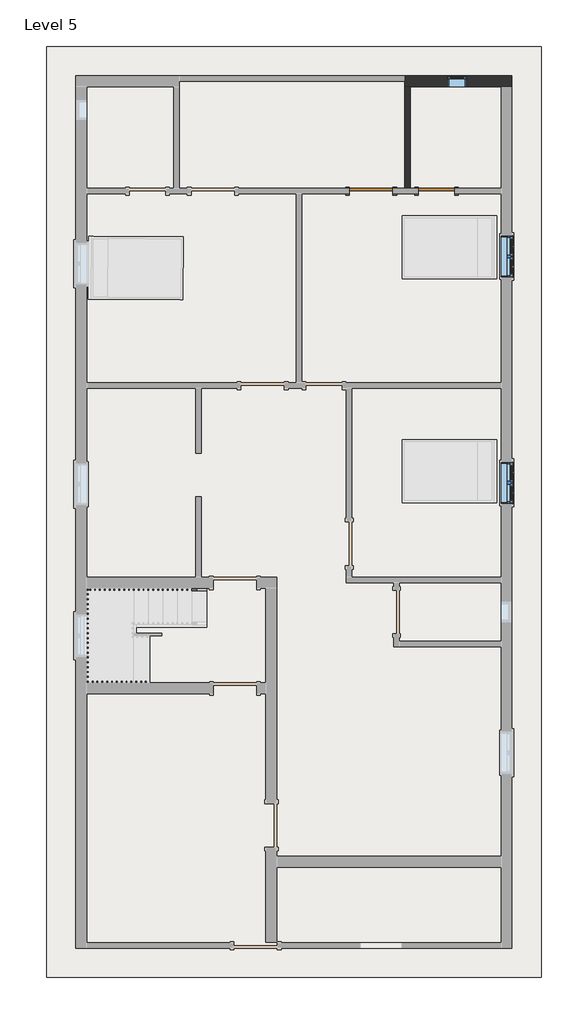
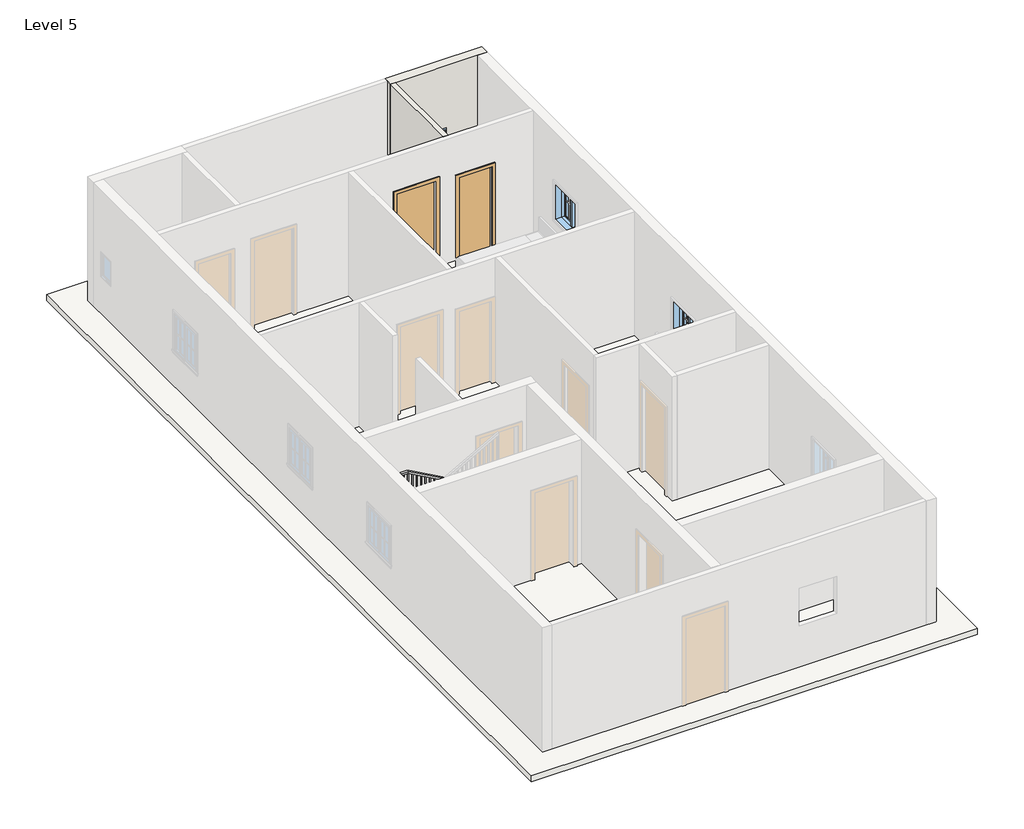
# One storey, part 2 of 3: 3 windows, 2 doors, 2 walls, 1 railing, 1 roof.
"""IFC4 building model written with IfcOpenShell, lengths in millimetres."""

from ifc_helpers import new_model, si_unit, frame, origin, place, context, project, spatial, polyline, outline, extrude, faceted_brep, transform, mapped, element, save
from components import door_f2b275c1, door_e5f9f3c4, window_aa618e30, window_339605e1

model = new_model("IFC4")

# Units and contexts
model_context = context("Model", 3, world=origin())
ifc_project = project(units=[si_unit("LENGTHUNIT", "METRE", prefix="MILLI")], contexts=[model_context])

# Site, building, storey
site = spatial("IfcSite", under=ifc_project)
building = spatial("IfcBuilding", under=site)
storey = spatial("IfcBuildingStorey", under=building, Name="Level 5", Elevation=9601.2)

# Doors
placement = place(None, origin())
door_shape = door_f2b275c1(model_context)
element("IfcDoor", 1, ObjectType="Single-Flush : 30\" x 80\"", at=placement, inside=storey, context=model_context, shape_type="MappedRepresentation", body=[
    mapped(door_shape, transform((1735.6084916, 8007.7072267, 9601.2), x_axis=(-1.0, 0.0, 0.0), y_axis=(0.0, -1.0, 0.0), z_axis=(0.0, 0.0, 1.0))),
])
door_2_shape = door_e5f9f3c4(model_context)
element("IfcDoor", 2, ObjectType="Single-Flush : 36\" x 84\"", at=placement, inside=storey, context=model_context, shape_type="MappedRepresentation", body=[
    mapped(door_2_shape, transform((364.0084916, 8007.7072267, 9601.2), x_axis=(1.0, 0.0, 0.0), y_axis=(0.0, 1.0, 0.0), z_axis=(0.0, 0.0, 1.0))),
])

# Railing
element("IfcRailing", 3, ObjectType="Handrail - Rectangular", at=placement, inside=storey, context=model_context, shape_type="SolidModel", body=[
    faceted_brep([(-3084.0415084, -367.9427733, 10684.9333333), (-3084.0415084, -367.9427733, 10626.820221), (-3084.0415084, -317.1427733, 10626.820221), (-3084.0415084, -317.1427733, 10684.9333333), (-4608.0415084, -367.9427733, 11531.6), (-4621.2051106, -367.9427733, 11480.8), (-4621.2051106, -317.1427733, 11480.8), (-4608.0415084, -317.1427733, 11531.6), (-5547.8415084, -367.9427733, 11531.6), (-5547.8415084, -367.9427733, 11480.8), (-5598.6415084, -317.1427733, 11480.8), (-5598.6415084, -317.1427733, 11531.6), (-5547.8415084, -2247.5427733, 11531.6), (-5547.8415084, -2247.5427733, 11480.8), (-5598.6415084, -2298.3427733, 11480.8), (-5598.6415084, -2298.3427733, 11531.6), (-4912.8415084, -2247.5427733, 11531.6), (-4899.6779062, -2247.5427733, 11480.8), (-4899.6779062, -2298.3427733, 11480.8), (-4912.8415084, -2298.3427733, 11531.6), (-3084.0415084, -2247.5427733, 12547.6), (-3084.0415084, -2298.3427733, 12547.6), (-3084.0415084, -2298.3427733, 12489.4868876), (-3084.0415084, -2247.5427733, 12489.4868876)], [[[0, 1, 2, 3]], [[1, 0, 4, 5]], [[2, 1, 5, 6]], [[3, 2, 6, 7]], [[0, 3, 7, 4]], [[5, 4, 8, 9]], [[6, 5, 9, 10]], [[7, 6, 10, 11]], [[4, 7, 11, 8]], [[9, 8, 12, 13]], [[10, 9, 13, 14]], [[11, 10, 14, 15]], [[8, 11, 15, 12]], [[13, 12, 16, 17]], [[14, 13, 17, 18]], [[15, 14, 18, 19]], [[12, 15, 19, 16]], [[20, 21, 22, 23]], [[17, 16, 20, 23]], [[18, 17, 23, 22]], [[19, 18, 22, 21]], [[16, 19, 21, 20]]]),
    extrude(outline(polyline([(12466.5563321, -3125.3165084), (12455.9729988, -3144.3665084), (11463.8666667, -3144.3665084), (11463.8666667, -3125.3165084), (12466.5563321, -3125.3165084)])), frame((0.0, -2282.4677733, 0.0), z_axis=(0.0, 1.0, 0.0), x_axis=(0.0, 0.0, 1.0)), (0.0, 0.0, 1.0), 19.05),
    extrude(outline(polyline([(12410.1118876, -3226.9165084), (12399.5285543, -3245.9665084), (11463.8666667, -3245.9665084), (11463.8666667, -3226.9165084), (12410.1118876, -3226.9165084)])), frame((0.0, -2282.4677733, 0.0), z_axis=(0.0, 1.0, 0.0), x_axis=(0.0, 0.0, 1.0)), (0.0, 0.0, 1.0), 19.05),
    extrude(outline(polyline([(12353.6674432, -3328.5165084), (12343.0841099, -3347.5665084), (11463.8666667, -3347.5665084), (11463.8666667, -3328.5165084), (12353.6674432, -3328.5165084)])), frame((0.0, -2282.4677733, 0.0), z_axis=(0.0, 1.0, 0.0), x_axis=(0.0, 0.0, 1.0)), (0.0, 0.0, 1.0), 19.05),
    extrude(outline(polyline([(12297.2229988, -3430.1165084), (12286.6396654, -3449.1665084), (11294.5333333, -3449.1665084), (11294.5333333, -3430.1165084), (12297.2229988, -3430.1165084)])), frame((0.0, -2282.4677733, 0.0), z_axis=(0.0, 1.0, 0.0), x_axis=(0.0, 0.0, 1.0)), (0.0, 0.0, 1.0), 19.05),
    extrude(outline(polyline([(12240.7785543, -3531.7165084), (12230.195221, -3550.7665084), (11294.5333333, -3550.7665084), (11294.5333333, -3531.7165084), (12240.7785543, -3531.7165084)])), frame((0.0, -2282.4677733, 0.0), z_axis=(0.0, 1.0, 0.0), x_axis=(0.0, 0.0, 1.0)), (0.0, 0.0, 1.0), 19.05),
    extrude(outline(polyline([(12184.3341099, -3633.3165084), (12173.7507765, -3652.3665084), (11294.5333333, -3652.3665084), (11294.5333333, -3633.3165084), (12184.3341099, -3633.3165084)])), frame((0.0, -2282.4677733, 0.0), z_axis=(0.0, 1.0, 0.0), x_axis=(0.0, 0.0, 1.0)), (0.0, 0.0, 1.0), 19.05),
    extrude(outline(polyline([(12127.8896654, -3734.9165084), (12117.3063321, -3753.9665084), (11125.2, -3753.9665084), (11125.2, -3734.9165084), (12127.8896654, -3734.9165084)])), frame((0.0, -2282.4677733, 0.0), z_axis=(0.0, 1.0, 0.0), x_axis=(0.0, 0.0, 1.0)), (0.0, 0.0, 1.0), 19.05),
    extrude(outline(polyline([(12071.445221, -3836.5165084), (12060.8618876, -3855.5665084), (11125.2, -3855.5665084), (11125.2, -3836.5165084), (12071.445221, -3836.5165084)])), frame((0.0, -2282.4677733, 0.0), z_axis=(0.0, 1.0, 0.0), x_axis=(0.0, 0.0, 1.0)), (0.0, 0.0, 1.0), 19.05),
    extrude(outline(polyline([(12015.0007765, -3938.1165084), (12004.4174432, -3957.1665084), (11125.2, -3957.1665084), (11125.2, -3938.1165084), (12015.0007765, -3938.1165084)])), frame((0.0, -2282.4677733, 0.0), z_axis=(0.0, 1.0, 0.0), x_axis=(0.0, 0.0, 1.0)), (0.0, 0.0, 1.0), 19.05),
    extrude(outline(polyline([(11958.5563321, -4039.7165084), (11947.9729988, -4058.7665084), (10955.8666667, -4058.7665084), (10955.8666667, -4039.7165084), (11958.5563321, -4039.7165084)])), frame((0.0, -2282.4677733, 0.0), z_axis=(0.0, 1.0, 0.0), x_axis=(0.0, 0.0, 1.0)), (0.0, 0.0, 1.0), 19.05),
    extrude(outline(polyline([(11902.1118876, -4141.3165084), (11891.5285543, -4160.3665084), (10955.8666667, -4160.3665084), (10955.8666667, -4141.3165084), (11902.1118876, -4141.3165084)])), frame((0.0, -2282.4677733, 0.0), z_axis=(0.0, 1.0, 0.0), x_axis=(0.0, 0.0, 1.0)), (0.0, 0.0, 1.0), 19.05),
    extrude(outline(polyline([(11845.6674432, -4242.9165084), (11835.0841099, -4261.9665084), (10955.8666667, -4261.9665084), (10955.8666667, -4242.9165084), (11845.6674432, -4242.9165084)])), frame((0.0, -2282.4677733, 0.0), z_axis=(0.0, 1.0, 0.0), x_axis=(0.0, 0.0, 1.0)), (0.0, 0.0, 1.0), 19.05),
    extrude(outline(polyline([(11789.2229988, -4344.5165084), (11778.6396654, -4363.5665084), (10786.5333333, -4363.5665084), (10786.5333333, -4344.5165084), (11789.2229988, -4344.5165084)])), frame((0.0, -2282.4677733, 0.0), z_axis=(0.0, 1.0, 0.0), x_axis=(0.0, 0.0, 1.0)), (0.0, 0.0, 1.0), 19.05),
    extrude(outline(polyline([(11732.7785543, -4446.1165084), (11722.195221, -4465.1665084), (10786.5333333, -4465.1665084), (10786.5333333, -4446.1165084), (11732.7785543, -4446.1165084)])), frame((0.0, -2282.4677733, 0.0), z_axis=(0.0, 1.0, 0.0), x_axis=(0.0, 0.0, 1.0)), (0.0, 0.0, 1.0), 19.05),
    extrude(outline(polyline([(11676.3341099, -4547.7165084), (11665.7507765, -4566.7665084), (10786.5333333, -4566.7665084), (10786.5333333, -4547.7165084), (11676.3341099, -4547.7165084)])), frame((0.0, -2282.4677733, 0.0), z_axis=(0.0, 1.0, 0.0), x_axis=(0.0, 0.0, 1.0)), (0.0, 0.0, 1.0), 19.05),
    extrude(outline(polyline([(11619.8896654, -4649.3165084), (11609.3063321, -4668.3665084), (10617.2, -4668.3665084), (10617.2, -4649.3165084), (11619.8896654, -4649.3165084)])), frame((0.0, -2282.4677733, 0.0), z_axis=(0.0, 1.0, 0.0), x_axis=(0.0, 0.0, 1.0)), (0.0, 0.0, 1.0), 19.05),
    extrude(outline(polyline([(11563.445221, -4750.9165084), (11552.8618876, -4769.9665084), (10617.2, -4769.9665084), (10617.2, -4750.9165084), (11563.445221, -4750.9165084)])), frame((0.0, -2282.4677733, 0.0), z_axis=(0.0, 1.0, 0.0), x_axis=(0.0, 0.0, 1.0)), (0.0, 0.0, 1.0), 19.05),
    extrude(outline(polyline([(11507.0007765, -4852.5165084), (11496.4174432, -4871.5665084), (10617.2, -4871.5665084), (10617.2, -4852.5165084), (11507.0007765, -4852.5165084)])), frame((0.0, -2282.4677733, 0.0), z_axis=(0.0, 1.0, 0.0), x_axis=(0.0, 0.0, 1.0)), (0.0, 0.0, 1.0), 19.05),
    extrude(outline(polyline([(-4973.1665084, -2282.4677733), (-4973.1665084, -2263.4177733), (-4954.1165084, -2263.4177733), (-4954.1165084, -2282.4677733), (-4973.1665084, -2282.4677733)])), frame((0.0, 0.0, 10617.2), z_axis=(0.0, 0.0, 1.0), x_axis=(1.0, 0.0, 0.0)), (0.0, 0.0, 1.0), 863.6),
    extrude(outline(polyline([(-5074.7665084, -2282.4677733), (-5074.7665084, -2263.4177733), (-5055.7165084, -2263.4177733), (-5055.7165084, -2282.4677733), (-5074.7665084, -2282.4677733)])), frame((0.0, 0.0, 10617.2), z_axis=(0.0, 0.0, 1.0), x_axis=(1.0, 0.0, 0.0)), (0.0, 0.0, 1.0), 863.6),
    extrude(outline(polyline([(-5176.3665084, -2282.4677733), (-5176.3665084, -2263.4177733), (-5157.3165084, -2263.4177733), (-5157.3165084, -2282.4677733), (-5176.3665084, -2282.4677733)])), frame((0.0, 0.0, 10617.2), z_axis=(0.0, 0.0, 1.0), x_axis=(1.0, 0.0, 0.0)), (0.0, 0.0, 1.0), 863.6),
    extrude(outline(polyline([(-5277.9665084, -2282.4677733), (-5277.9665084, -2263.4177733), (-5258.9165084, -2263.4177733), (-5258.9165084, -2282.4677733), (-5277.9665084, -2282.4677733)])), frame((0.0, 0.0, 10617.2), z_axis=(0.0, 0.0, 1.0), x_axis=(1.0, 0.0, 0.0)), (0.0, 0.0, 1.0), 863.6),
    extrude(outline(polyline([(-5379.5665084, -2282.4677733), (-5379.5665084, -2263.4177733), (-5360.5165084, -2263.4177733), (-5360.5165084, -2282.4677733), (-5379.5665084, -2282.4677733)])), frame((0.0, 0.0, 10617.2), z_axis=(0.0, 0.0, 1.0), x_axis=(1.0, 0.0, 0.0)), (0.0, 0.0, 1.0), 863.6),
    extrude(outline(polyline([(-5481.1665084, -2282.4677733), (-5481.1665084, -2263.4177733), (-5462.1165084, -2263.4177733), (-5462.1165084, -2282.4677733), (-5481.1665084, -2282.4677733)])), frame((0.0, 0.0, 10617.2), z_axis=(0.0, 0.0, 1.0), x_axis=(1.0, 0.0, 0.0)), (0.0, 0.0, 1.0), 863.6),
    extrude(outline(polyline([(-5582.7665084, -2161.8177733), (-5563.7165084, -2161.8177733), (-5563.7165084, -2180.8677733), (-5582.7665084, -2180.8677733), (-5582.7665084, -2161.8177733)])), frame((0.0, 0.0, 10617.2), z_axis=(0.0, 0.0, 1.0), x_axis=(1.0, 0.0, 0.0)), (0.0, 0.0, 1.0), 863.6),
    extrude(outline(polyline([(-5582.7665084, -2060.2177733), (-5563.7165084, -2060.2177733), (-5563.7165084, -2079.2677733), (-5582.7665084, -2079.2677733), (-5582.7665084, -2060.2177733)])), frame((0.0, 0.0, 10617.2), z_axis=(0.0, 0.0, 1.0), x_axis=(1.0, 0.0, 0.0)), (0.0, 0.0, 1.0), 863.6),
    extrude(outline(polyline([(-5582.7665084, -1958.6177733), (-5563.7165084, -1958.6177733), (-5563.7165084, -1977.6677733), (-5582.7665084, -1977.6677733), (-5582.7665084, -1958.6177733)])), frame((0.0, 0.0, 10617.2), z_axis=(0.0, 0.0, 1.0), x_axis=(1.0, 0.0, 0.0)), (0.0, 0.0, 1.0), 863.6),
    extrude(outline(polyline([(-5582.7665084, -1857.0177733), (-5563.7165084, -1857.0177733), (-5563.7165084, -1876.0677733), (-5582.7665084, -1876.0677733), (-5582.7665084, -1857.0177733)])), frame((0.0, 0.0, 10617.2), z_axis=(0.0, 0.0, 1.0), x_axis=(1.0, 0.0, 0.0)), (0.0, 0.0, 1.0), 863.6),
    extrude(outline(polyline([(-5582.7665084, -1755.4177733), (-5563.7165084, -1755.4177733), (-5563.7165084, -1774.4677733), (-5582.7665084, -1774.4677733), (-5582.7665084, -1755.4177733)])), frame((0.0, 0.0, 10617.2), z_axis=(0.0, 0.0, 1.0), x_axis=(1.0, 0.0, 0.0)), (0.0, 0.0, 1.0), 863.6),
    extrude(outline(polyline([(-5582.7665084, -1653.8177733), (-5563.7165084, -1653.8177733), (-5563.7165084, -1672.8677733), (-5582.7665084, -1672.8677733), (-5582.7665084, -1653.8177733)])), frame((0.0, 0.0, 10617.2), z_axis=(0.0, 0.0, 1.0), x_axis=(1.0, 0.0, 0.0)), (0.0, 0.0, 1.0), 863.6),
    extrude(outline(polyline([(-5582.7665084, -1552.2177733), (-5563.7165084, -1552.2177733), (-5563.7165084, -1571.2677733), (-5582.7665084, -1571.2677733), (-5582.7665084, -1552.2177733)])), frame((0.0, 0.0, 10617.2), z_axis=(0.0, 0.0, 1.0), x_axis=(1.0, 0.0, 0.0)), (0.0, 0.0, 1.0), 863.6),
    extrude(outline(polyline([(-5582.7665084, -1450.6177733), (-5563.7165084, -1450.6177733), (-5563.7165084, -1469.6677733), (-5582.7665084, -1469.6677733), (-5582.7665084, -1450.6177733)])), frame((0.0, 0.0, 10617.2), z_axis=(0.0, 0.0, 1.0), x_axis=(1.0, 0.0, 0.0)), (0.0, 0.0, 1.0), 863.6),
    extrude(outline(polyline([(-5582.7665084, -1349.0177733), (-5563.7165084, -1349.0177733), (-5563.7165084, -1368.0677733), (-5582.7665084, -1368.0677733), (-5582.7665084, -1349.0177733)])), frame((0.0, 0.0, 10617.2), z_axis=(0.0, 0.0, 1.0), x_axis=(1.0, 0.0, 0.0)), (0.0, 0.0, 1.0), 863.6),
    extrude(outline(polyline([(-5582.7665084, -1247.4177733), (-5563.7165084, -1247.4177733), (-5563.7165084, -1266.4677733), (-5582.7665084, -1266.4677733), (-5582.7665084, -1247.4177733)])), frame((0.0, 0.0, 10617.2), z_axis=(0.0, 0.0, 1.0), x_axis=(1.0, 0.0, 0.0)), (0.0, 0.0, 1.0), 863.6),
    extrude(outline(polyline([(-5582.7665084, -1145.8177733), (-5563.7165084, -1145.8177733), (-5563.7165084, -1164.8677733), (-5582.7665084, -1164.8677733), (-5582.7665084, -1145.8177733)])), frame((0.0, 0.0, 10617.2), z_axis=(0.0, 0.0, 1.0), x_axis=(1.0, 0.0, 0.0)), (0.0, 0.0, 1.0), 863.6),
    extrude(outline(polyline([(-5582.7665084, -1044.2177733), (-5563.7165084, -1044.2177733), (-5563.7165084, -1063.2677733), (-5582.7665084, -1063.2677733), (-5582.7665084, -1044.2177733)])), frame((0.0, 0.0, 10617.2), z_axis=(0.0, 0.0, 1.0), x_axis=(1.0, 0.0, 0.0)), (0.0, 0.0, 1.0), 863.6),
    extrude(outline(polyline([(-5582.7665084, -942.6177733), (-5563.7165084, -942.6177733), (-5563.7165084, -961.6677733), (-5582.7665084, -961.6677733), (-5582.7665084, -942.6177733)])), frame((0.0, 0.0, 10617.2), z_axis=(0.0, 0.0, 1.0), x_axis=(1.0, 0.0, 0.0)), (0.0, 0.0, 1.0), 863.6),
    extrude(outline(polyline([(-5582.7665084, -841.0177733), (-5563.7165084, -841.0177733), (-5563.7165084, -860.0677733), (-5582.7665084, -860.0677733), (-5582.7665084, -841.0177733)])), frame((0.0, 0.0, 10617.2), z_axis=(0.0, 0.0, 1.0), x_axis=(1.0, 0.0, 0.0)), (0.0, 0.0, 1.0), 863.6),
    extrude(outline(polyline([(-5582.7665084, -739.4177733), (-5563.7165084, -739.4177733), (-5563.7165084, -758.4677733), (-5582.7665084, -758.4677733), (-5582.7665084, -739.4177733)])), frame((0.0, 0.0, 10617.2), z_axis=(0.0, 0.0, 1.0), x_axis=(1.0, 0.0, 0.0)), (0.0, 0.0, 1.0), 863.6),
    extrude(outline(polyline([(-5582.7665084, -637.8177733), (-5563.7165084, -637.8177733), (-5563.7165084, -656.8677733), (-5582.7665084, -656.8677733), (-5582.7665084, -637.8177733)])), frame((0.0, 0.0, 10617.2), z_axis=(0.0, 0.0, 1.0), x_axis=(1.0, 0.0, 0.0)), (0.0, 0.0, 1.0), 863.6),
    extrude(outline(polyline([(-5582.7665084, -536.2177733), (-5563.7165084, -536.2177733), (-5563.7165084, -555.2677733), (-5582.7665084, -555.2677733), (-5582.7665084, -536.2177733)])), frame((0.0, 0.0, 10617.2), z_axis=(0.0, 0.0, 1.0), x_axis=(1.0, 0.0, 0.0)), (0.0, 0.0, 1.0), 863.6),
    extrude(outline(polyline([(-5582.7665084, -434.6177733), (-5563.7165084, -434.6177733), (-5563.7165084, -453.6677733), (-5582.7665084, -453.6677733), (-5582.7665084, -434.6177733)])), frame((0.0, 0.0, 10617.2), z_axis=(0.0, 0.0, 1.0), x_axis=(1.0, 0.0, 0.0)), (0.0, 0.0, 1.0), 863.6),
    extrude(outline(polyline([(-5512.9165084, -333.0177733), (-5512.9165084, -352.0677733), (-5531.9665084, -352.0677733), (-5531.9665084, -333.0177733), (-5512.9165084, -333.0177733)])), frame((0.0, 0.0, 10617.2), z_axis=(0.0, 0.0, 1.0), x_axis=(1.0, 0.0, 0.0)), (0.0, 0.0, 1.0), 863.6),
    extrude(outline(polyline([(-5411.3165084, -333.0177733), (-5411.3165084, -352.0677733), (-5430.3665084, -352.0677733), (-5430.3665084, -333.0177733), (-5411.3165084, -333.0177733)])), frame((0.0, 0.0, 10617.2), z_axis=(0.0, 0.0, 1.0), x_axis=(1.0, 0.0, 0.0)), (0.0, 0.0, 1.0), 863.6),
    extrude(outline(polyline([(-5309.7165084, -333.0177733), (-5309.7165084, -352.0677733), (-5328.7665084, -352.0677733), (-5328.7665084, -333.0177733), (-5309.7165084, -333.0177733)])), frame((0.0, 0.0, 10617.2), z_axis=(0.0, 0.0, 1.0), x_axis=(1.0, 0.0, 0.0)), (0.0, 0.0, 1.0), 863.6),
    extrude(outline(polyline([(-5208.1165084, -333.0177733), (-5208.1165084, -352.0677733), (-5227.1665084, -352.0677733), (-5227.1665084, -333.0177733), (-5208.1165084, -333.0177733)])), frame((0.0, 0.0, 10617.2), z_axis=(0.0, 0.0, 1.0), x_axis=(1.0, 0.0, 0.0)), (0.0, 0.0, 1.0), 863.6),
    extrude(outline(polyline([(-5106.5165084, -333.0177733), (-5106.5165084, -352.0677733), (-5125.5665084, -352.0677733), (-5125.5665084, -333.0177733), (-5106.5165084, -333.0177733)])), frame((0.0, 0.0, 10617.2), z_axis=(0.0, 0.0, 1.0), x_axis=(1.0, 0.0, 0.0)), (0.0, 0.0, 1.0), 863.6),
    extrude(outline(polyline([(-5004.9165084, -333.0177733), (-5004.9165084, -352.0677733), (-5023.9665084, -352.0677733), (-5023.9665084, -333.0177733), (-5004.9165084, -333.0177733)])), frame((0.0, 0.0, 10617.2), z_axis=(0.0, 0.0, 1.0), x_axis=(1.0, 0.0, 0.0)), (0.0, 0.0, 1.0), 863.6),
    extrude(outline(polyline([(-4903.3165084, -333.0177733), (-4903.3165084, -352.0677733), (-4922.3665084, -352.0677733), (-4922.3665084, -333.0177733), (-4903.3165084, -333.0177733)])), frame((0.0, 0.0, 10617.2), z_axis=(0.0, 0.0, 1.0), x_axis=(1.0, 0.0, 0.0)), (0.0, 0.0, 1.0), 863.6),
    extrude(outline(polyline([(-4801.7165084, -333.0177733), (-4801.7165084, -352.0677733), (-4820.7665084, -352.0677733), (-4820.7665084, -333.0177733), (-4801.7165084, -333.0177733)])), frame((0.0, 0.0, 10617.2), z_axis=(0.0, 0.0, 1.0), x_axis=(1.0, 0.0, 0.0)), (0.0, 0.0, 1.0), 863.6),
    extrude(outline(polyline([(-4700.1165084, -333.0177733), (-4700.1165084, -352.0677733), (-4719.1665084, -352.0677733), (-4719.1665084, -333.0177733), (-4700.1165084, -333.0177733)])), frame((0.0, 0.0, 10617.2), z_axis=(0.0, 0.0, 1.0), x_axis=(1.0, 0.0, 0.0)), (0.0, 0.0, 1.0), 863.6),
    extrude(outline(polyline([(11468.195221, -4598.5165084), (11478.7785543, -4617.5665084), (10617.2, -4617.5665084), (10617.2, -4598.5165084), (11468.195221, -4598.5165084)])), frame((0.0, -352.0677733, 0.0), z_axis=(0.0, 1.0, 0.0), x_axis=(0.0, 0.0, 1.0)), (0.0, 0.0, 1.0), 19.05),
    extrude(outline(polyline([(11411.7507765, -4496.9165084), (11422.3341099, -4515.9665084), (10447.8666667, -4515.9665084), (10447.8666667, -4496.9165084), (11411.7507765, -4496.9165084)])), frame((0.0, -352.0677733, 0.0), z_axis=(0.0, 1.0, 0.0), x_axis=(0.0, 0.0, 1.0)), (0.0, 0.0, 1.0), 19.05),
    extrude(outline(polyline([(11355.3063321, -4395.3165084), (11365.8896654, -4414.3665084), (10447.8666667, -4414.3665084), (10447.8666667, -4395.3165084), (11355.3063321, -4395.3165084)])), frame((0.0, -352.0677733, 0.0), z_axis=(0.0, 1.0, 0.0), x_axis=(0.0, 0.0, 1.0)), (0.0, 0.0, 1.0), 19.05),
    extrude(outline(polyline([(11298.8618876, -4293.7165084), (11309.445221, -4312.7665084), (10447.8666667, -4312.7665084), (10447.8666667, -4293.7165084), (11298.8618876, -4293.7165084)])), frame((0.0, -352.0677733, 0.0), z_axis=(0.0, 1.0, 0.0), x_axis=(0.0, 0.0, 1.0)), (0.0, 0.0, 1.0), 19.05),
    extrude(outline(polyline([(11242.4174432, -4192.1165084), (11253.0007765, -4211.1665084), (10278.5333333, -4211.1665084), (10278.5333333, -4192.1165084), (11242.4174432, -4192.1165084)])), frame((0.0, -352.0677733, 0.0), z_axis=(0.0, 1.0, 0.0), x_axis=(0.0, 0.0, 1.0)), (0.0, 0.0, 1.0), 19.05),
    extrude(outline(polyline([(11185.9729988, -4090.5165084), (11196.5563321, -4109.5665084), (10278.5333333, -4109.5665084), (10278.5333333, -4090.5165084), (11185.9729988, -4090.5165084)])), frame((0.0, -352.0677733, 0.0), z_axis=(0.0, 1.0, 0.0), x_axis=(0.0, 0.0, 1.0)), (0.0, 0.0, 1.0), 19.05),
    extrude(outline(polyline([(11129.5285543, -3988.9165084), (11140.1118876, -4007.9665084), (10278.5333333, -4007.9665084), (10278.5333333, -3988.9165084), (11129.5285543, -3988.9165084)])), frame((0.0, -352.0677733, 0.0), z_axis=(0.0, 1.0, 0.0), x_axis=(0.0, 0.0, 1.0)), (0.0, 0.0, 1.0), 19.05),
    extrude(outline(polyline([(11073.0841099, -3887.3165084), (11083.6674432, -3906.3665084), (10109.2, -3906.3665084), (10109.2, -3887.3165084), (11073.0841099, -3887.3165084)])), frame((0.0, -352.0677733, 0.0), z_axis=(0.0, 1.0, 0.0), x_axis=(0.0, 0.0, 1.0)), (0.0, 0.0, 1.0), 19.05),
    extrude(outline(polyline([(11016.6396654, -3785.7165084), (11027.2229988, -3804.7665084), (10109.2, -3804.7665084), (10109.2, -3785.7165084), (11016.6396654, -3785.7165084)])), frame((0.0, -352.0677733, 0.0), z_axis=(0.0, 1.0, 0.0), x_axis=(0.0, 0.0, 1.0)), (0.0, 0.0, 1.0), 19.05),
    extrude(outline(polyline([(10960.195221, -3684.1165084), (10970.7785543, -3703.1665084), (10109.2, -3703.1665084), (10109.2, -3684.1165084), (10960.195221, -3684.1165084)])), frame((0.0, -352.0677733, 0.0), z_axis=(0.0, 1.0, 0.0), x_axis=(0.0, 0.0, 1.0)), (0.0, 0.0, 1.0), 19.05),
    extrude(outline(polyline([(10903.7507765, -3582.5165084), (10914.3341099, -3601.5665084), (9939.8666667, -3601.5665084), (9939.8666667, -3582.5165084), (10903.7507765, -3582.5165084)])), frame((0.0, -352.0677733, 0.0), z_axis=(0.0, 1.0, 0.0), x_axis=(0.0, 0.0, 1.0)), (0.0, 0.0, 1.0), 19.05),
    extrude(outline(polyline([(10847.3063321, -3480.9165084), (10857.8896654, -3499.9665084), (9939.8666667, -3499.9665084), (9939.8666667, -3480.9165084), (10847.3063321, -3480.9165084)])), frame((0.0, -352.0677733, 0.0), z_axis=(0.0, 1.0, 0.0), x_axis=(0.0, 0.0, 1.0)), (0.0, 0.0, 1.0), 19.05),
    extrude(outline(polyline([(10790.8618876, -3379.3165084), (10801.445221, -3398.3665084), (9939.8666667, -3398.3665084), (9939.8666667, -3379.3165084), (10790.8618876, -3379.3165084)])), frame((0.0, -352.0677733, 0.0), z_axis=(0.0, 1.0, 0.0), x_axis=(0.0, 0.0, 1.0)), (0.0, 0.0, 1.0), 19.05),
    extrude(outline(polyline([(10734.4174432, -3277.7165084), (10745.0007765, -3296.7665084), (9770.5333333, -3296.7665084), (9770.5333333, -3277.7165084), (10734.4174432, -3277.7165084)])), frame((0.0, -352.0677733, 0.0), z_axis=(0.0, 1.0, 0.0), x_axis=(0.0, 0.0, 1.0)), (0.0, 0.0, 1.0), 19.05),
    extrude(outline(polyline([(10677.9729988, -3176.1165084), (10688.5563321, -3195.1665084), (9770.5333333, -3195.1665084), (9770.5333333, -3176.1165084), (10677.9729988, -3176.1165084)])), frame((0.0, -352.0677733, 0.0), z_axis=(0.0, 1.0, 0.0), x_axis=(0.0, 0.0, 1.0)), (0.0, 0.0, 1.0), 19.05),
    extrude(outline(polyline([(-5582.7665084, -2263.4177733), (-5563.7165084, -2263.4177733), (-5563.7165084, -2282.4677733), (-5582.7665084, -2282.4677733), (-5582.7665084, -2263.4177733)])), frame((0.0, 0.0, 10617.2), z_axis=(0.0, 0.0, 1.0), x_axis=(1.0, 0.0, 0.0)), (0.0, 0.0, 1.0), 863.6),
    extrude(outline(polyline([(-5563.7165084, -333.0177733), (-5563.7165084, -352.0677733), (-5582.7665084, -352.0677733), (-5582.7665084, -333.0177733), (-5563.7165084, -333.0177733)])), frame((0.0, 0.0, 10617.2), z_axis=(0.0, 0.0, 1.0), x_axis=(1.0, 0.0, 0.0)), (0.0, 0.0, 1.0), 863.6),
    extrude(outline(polyline([(12489.4868876, -3084.0415084), (12478.9035543, -3103.0915084), (11463.8666667, -3103.0915084), (11463.8666667, -3084.0415084), (12489.4868876, -3084.0415084)])), frame((0.0, -2282.4677733, 0.0), z_axis=(0.0, 1.0, 0.0), x_axis=(0.0, 0.0, 1.0)), (0.0, 0.0, 1.0), 19.05),
    extrude(outline(polyline([(10626.820221, -3084.0415084), (10637.4035543, -3103.0915084), (9770.5333333, -3103.0915084), (9770.5333333, -3084.0415084), (10626.820221, -3084.0415084)])), frame((0.0, -352.0677733, 0.0), z_axis=(0.0, 1.0, 0.0), x_axis=(0.0, 0.0, 1.0)), (0.0, 0.0, 1.0), 19.05),
])

# Roof
element("IfcRoof", 4, ObjectType="Generic - 12\"", at=placement, inside=storey, context=model_context, shape_type="SweptSolid", body=[
    extrude(outline(polyline([(-6436.8415084, 11036.6572267), (3926.3584916, 11036.6572267), (3926.3584916, -8470.5427733), (-6436.8415084, -8470.5427733), (-6436.8415084, 11036.6572267)])), frame((0.0, 0.0, 9448.8), z_axis=(0.0, 0.0, 1.0), x_axis=(1.0, 0.0, 0.0)), (0.0, 0.0, 1.0), 152.4),
])

# Walls
element("IfcWall", 5, ObjectType="WALL4.5\"", at=placement, inside=storey, context=model_context, shape_type="SweptSolid", body=[
    extrude(outline(polyline([(1068.8584916, 8064.8572267), (1068.8584916, 10198.4572267), (1183.1584916, 10198.4572267), (1183.1584916, 8064.8572267), (1068.8584916, 8064.8572267)])), frame((0.0, 0.0, 9601.2), z_axis=(0.0, 0.0, 1.0), x_axis=(1.0, 0.0, 0.0)), (0.0, 0.0, 1.0), 3048.0),
])
element("IfcWall", 6, ObjectType="WALL9\"", at=placement, inside=storey, context=model_context, shape_type="Brep", body=[
    faceted_brep([(1068.8584916, 10198.4572267, 9601.2), (1183.1584916, 10198.4572267, 9601.2), (3088.1584916, 10198.4572267, 9601.2), (3316.7584916, 10198.4572267, 9601.2), (3316.7584916, 10198.4572267, 12649.2), (3088.1584916, 10198.4572267, 12649.2), (1183.1584916, 10198.4572267, 12649.2), (1068.8584916, 10198.4572267, 12649.2), (2367.4334916, 10198.4572267, 11125.2), (2367.4334916, 10198.4572267, 10515.6), (1961.0334916, 10198.4572267, 10515.6), (1961.0334916, 10198.4572267, 11125.2), (1068.8584916, 10427.0572267, 9601.2), (1068.8584916, 10427.0572267, 12649.2), (3316.7584916, 10427.0572267, 12649.2), (3316.7584916, 10427.0572267, 9601.2), (2367.4334916, 10427.0572267, 11125.2), (1961.0334916, 10427.0572267, 11125.2), (1961.0334916, 10427.0572267, 10515.6), (2367.4334916, 10427.0572267, 10515.6), (1068.8584916, 10312.7572267, 9601.2), (1068.8584916, 10312.7572267, 12649.2)], [[[0, 1, 2, 3, 4, 5, 6, 7], [8, 9, 10, 11]], [[12, 13, 14, 15], [16, 17, 18, 19]], [[3, 2, 1, 0, 20, 12, 15]], [[4, 3, 15, 14]], [[0, 7, 21, 13, 12, 20]], [[9, 8, 16, 19]], [[10, 9, 19, 18]], [[11, 10, 18, 17]], [[8, 11, 17, 16]], [[7, 6, 5, 4, 14, 13, 21]]]),
])

# Windows
window_shape = window_aa618e30(model_context)
element("IfcWindow", 7, ObjectType="Fixed : 16\" x 24\"", at=placement, inside=storey, context=model_context, shape_type="MappedRepresentation", body=[
    mapped(window_shape, transform((2202.3334916, 10312.7572267, 9601.2), x_axis=(1.0, 0.0, 0.0), y_axis=(0.0, 1.0, 0.0), z_axis=(0.0, 0.0, 1.0))),
])
window_2_shape = window_339605e1(model_context)
element("IfcWindow", 8, ObjectType="Window-Casement-Double : 34\" x 36\"", at=placement, inside=storey, context=model_context, shape_type="MappedRepresentation", body=[
    mapped(window_2_shape, transform((3202.4584916, 6636.1072267, 9601.2), x_axis=(0.0, -1.0, 0.0), y_axis=(1.0, 0.0, 0.0), z_axis=(0.0, 0.0, 1.0))),
])
element("IfcWindow", 9, ObjectType="Window-Casement-Double : 34\" x 36\"", at=placement, inside=storey, context=model_context, shape_type="MappedRepresentation", body=[
    mapped(window_2_shape, transform((3202.4584916, 1892.6572267, 9601.2), x_axis=(0.0, -1.0, 0.0), y_axis=(1.0, 0.0, 0.0), z_axis=(0.0, 0.0, 1.0))),
])

save(model, "model.ifc")

# Revit data of these elements
# Type "Single-Flush : 30\" x 80\""
#   Type Mark = "5"
#   Construction Type Id = "MDOOR"
#   Assembly Code = "C1020"
#   Analytic Construction = "Metal"
#   Thickness = 0' - 2"
#   Heat Transfer Coefficient (U) = 0.651978 BTU/(h·ft²·°F)
#   Height = 6' - 8"
#   Trim Projection Ext = 0' - 1"
#   Trim Projection Int = 0' - 1"
#   Trim Width = 0' - 3"
#   Width = 2' - 6"
#   Define Thermal Properties by = 1
#   Define Thermal Properties by = 1
#   Door Material = Door - Panel
#   Frame Material = Door - Frame
#   Visual Light Transmittance = 0
#   Solar Heat Gain Coefficient = 0
#   Function = (empty or 0)
#   Wall Closure = (empty or 0)
# Type "Single-Flush : 36\" x 84\""
#   Type Mark = "1"
#   Construction Type Id = "MDOOR"
#   Assembly Code = "C1020"
#   Analytic Construction = "Metal"
#   Thickness = 0' - 2"
#   Heat Transfer Coefficient (U) = 0.651978 BTU/(h·ft²·°F)
#   Height = 7' - 0"
#   Trim Projection Ext = 0' - 1"
#   Trim Projection Int = 0' - 1"
#   Trim Width = 0' - 3"
#   Width = 3' - 0"
#   Define Thermal Properties by = 1
#   Define Thermal Properties by = 1
#   Door Material = Door - Panel
#   Frame Material = Door - Frame
#   Visual Light Transmittance = 0
#   Solar Heat Gain Coefficient = 0
#   Function = (empty or 0)
#   Wall Closure = (empty or 0)
# Type "Handrail - Rectangular"
#   Assembly Code = "C2010400"
#   built-in parameter 1008612 = 0.0416667 (stored number, unit not read)
#   built-in parameter 1008611 = 0.0416667 (stored number, unit not read)
#   built-in parameter 1008609 = 0.333333 (stored number, unit not read)
#   built-in parameter 1008604 = 0.166667 (stored number, unit not read)
#   built-in parameter 1008603 = 0.166667 (stored number, unit not read)
#   Railing Height = 3' - 0"
#   built-in parameter 1008630 = 2
#   built-in parameter 1008610 = 2
#   built-in parameter 1008618 = Baluster - Square : 3/4"
# Type "Generic - 12\""
#   Assembly Code = "B1020"
#   Layers, outside or top first: 0' - 6" no material (function 1)
# Type "WALL4.5\""
#   Assembly Code = "B2010"
#   Layers, outside or top first: 0' - 4 1/2" no material (function 1)
# Type "WALL9\""
#   Assembly Code = "B2010"
#   Layers, outside or top first: 0' - 9" no material (function 1)
# Type "Fixed : 16\" x 24\""
#   Type Mark = "4"
#   Construction Type Id = "GSP4R"
#   Assembly Code = "B2020100"
#   Analytic Construction = "1/8 in Pilkington single glazing"
#   Visual Light Transmittance = 0.9
#   Solar Heat Gain Coefficient = 0.78
#   Heat Transfer Coefficient (U) = 0.6496 BTU/(h·ft²·°F)
#   Height = 2' - 0"
#   Default Sill Height = 3' - 0"
#   Width = 1' - 4"
#   Window Inset = 0' - 0 3/4"
#   Define Thermal Properties by = 1
#   Define Thermal Properties by = 1
#   Glass Pane Material = Glass
#   Sash Material = Sash
#   Wall Closure = (empty or 0)
# Type "Window-Casement-Double : 34\" x 36\""
#   Type Mark = "14"
#   Fire Rating = "0.5h"
#   Assembly Code = "B2020100"
#   Analytic Construction = "Double glazing - domestic"
#   Frame Extension [instance default] = 0' - 0 1/4"
#   Window Inset [instance default] = 0' - 0"
#   Wall Thickness [instance default] = 0' - 6"
#   Interior Wall Closure [instance default] = 0' - 2 1/4"
#   Half Width = 1' - 5"
#   Visual Light Transmittance = 0.81
#   Thermal Resistance (R) = 1.8146 (h·ft²·°F)/BTU
#   Solar Heat Gain Coefficient = 0.76
#   Rough Width = 2' - 10 1/2"
#   Rough Height = 3' - 0 1/2"
#   Height = 3' - 0"
#   Heat Transfer Coefficient (U) = 0.5511 BTU/(h·ft²·°F)
#   Exterior Wall Closure [instance default] = 0' - 1 1/4"
#   Extension Jamb [instance default] = 0' - 2 1/4"
#   Default Sill Height = 3' - 0"
#   Width = 2' - 10"
#   Define Thermal Properties by = 0
#   Muntin Visibility = yes
#   Interior Trim Visibility [instance default] = yes
#   Exterior Trim Visibility [instance default] = yes
#   Extension Jamb Visibility [instance default] = yes
#   Interior Trim Material = Wood - Stained
#   Muntin Pattern = Muntin Pattern_2x2 : Muntin Pattern_2x2
#   Interior Trim = Trim-Window-Interior-Flat : Picture Frame
#   Interior Frame Material = Wood - Stained
#   Glass Panel Material = Glass
#   Exterior Trim Material = Clad - White
#   Exterior Trim = Trim-Window-Exterior-Flat : with Sill
#   Exterior Frame Material = Clad - White
#   Wall Closure = (empty or 0)
# Element 1 (IfcDoor, "Single-Flush : 30\" x 80\"")
#   Phase Created = New Construction
#   Materials on its faces: "Door - Frame", "Door - Panel"
# Element 2 (IfcDoor, "Single-Flush : 36\" x 84\"")
#   Phase Created = New Construction
#   Materials on its faces: "Door - Frame", "Door - Panel"
# Element 3 (IfcRailing, "Handrail - Rectangular")
#   Phase Created = New Construction
# Element 4 (IfcRoof, "Generic - 12\"")
#   built-in parameter 1001705 = 31.5 (stored number, unit not read)
#   built-in parameter 1001701 = -0.5 (stored number, unit not read)
#   built-in parameter 1001710 = 33615
#   Phase Created = New Construction
#   Materials on its faces: "Default Roof", "Wood Planks"
# Element 5 (IfcWall, "WALL4.5\"")
#   Top Offset = 0' - 0"
#   Base Offset = 0' - 0"
#   Unconnected Height = 10' - 0"
#   wall height = 10' - 0"
#   Phase Created = New Construction
#   Base Constraint = Level 5
#   Materials on its faces: "Default Wall", "Wood Planks"
# Element 6 (IfcWall, "WALL9\"")
#   Top Offset = 0' - 0"
#   Base Offset = 0' - 0"
#   Unconnected Height = 10' - 0"
#   wall height = 10' - 0"
#   Phase Created = New Construction
#   Base Constraint = Level 5
#   Materials on its faces: "Default Wall", "Wood Planks"
# Element 7 (IfcWindow, "Fixed : 16\" x 24\"")
#   Mark = "29"
#   Phase Created = New Construction
#   Materials on its faces: "Sash", "Glass"
# Element 8 (IfcWindow, "Window-Casement-Double : 34\" x 36\"")
#   Mark = "31"
#   Window Inset = 0' - 0"
#   Interior Wall Closure = 0' - 2 1/4"
#   Frame Extension = 0' - 0 1/4"
#   Exterior Wall Closure = 0' - 1 1/4"
#   Interior Trim Visibility = yes
#   Exterior Trim Visibility = yes
#   Phase Created = New Construction
#   Materials on its faces: "Wood - Stained", "Glass", "Clad - White"
# Element 9 (IfcWindow, "Window-Casement-Double : 34\" x 36\"")
#   Mark = "32"
#   Window Inset = 0' - 0"
#   Interior Wall Closure = 0' - 2 1/4"
#   Frame Extension = 0' - 0 1/4"
#   Exterior Wall Closure = 0' - 1 1/4"
#   Interior Trim Visibility = yes
#   Exterior Trim Visibility = yes
#   Phase Created = New Construction
#   Materials on its faces: "Wood - Stained", "Glass", "Clad - White"
# Materials
#   "Door - Panel": class "Wood", colour RGB 210 159 95, transparency 0, Cost = 0
#   "Door - Frame": colour RGB 118 70 51, transparency 0, Cost = 0
#   "Glass": class "Glass", colour RGB 0 128 192, transparency 0.75, Description = "Soda Lime Glass", Cost = 0
#   "Sash": class "Wood", colour RGB 224 178 126, transparency 0, Cost = 0
#   "Wood - Stained": class "Wood", colour RGB 224 178 126, transparency 0, Cost = 0
#   "Clad - White": class "Wood", colour RGB 242 242 238, transparency 0, Cost = 0
#   "Default Roof": colour RGB 88 101 114, transparency 0, Cost = 0
#   "Wood Planks": class "Wood", colour RGB 193 160 115, transparency 0, Description = "Physical material.", Cost = 0
#   "Default Wall": colour RGB 128 128 128, transparency 0, Cost = 0
